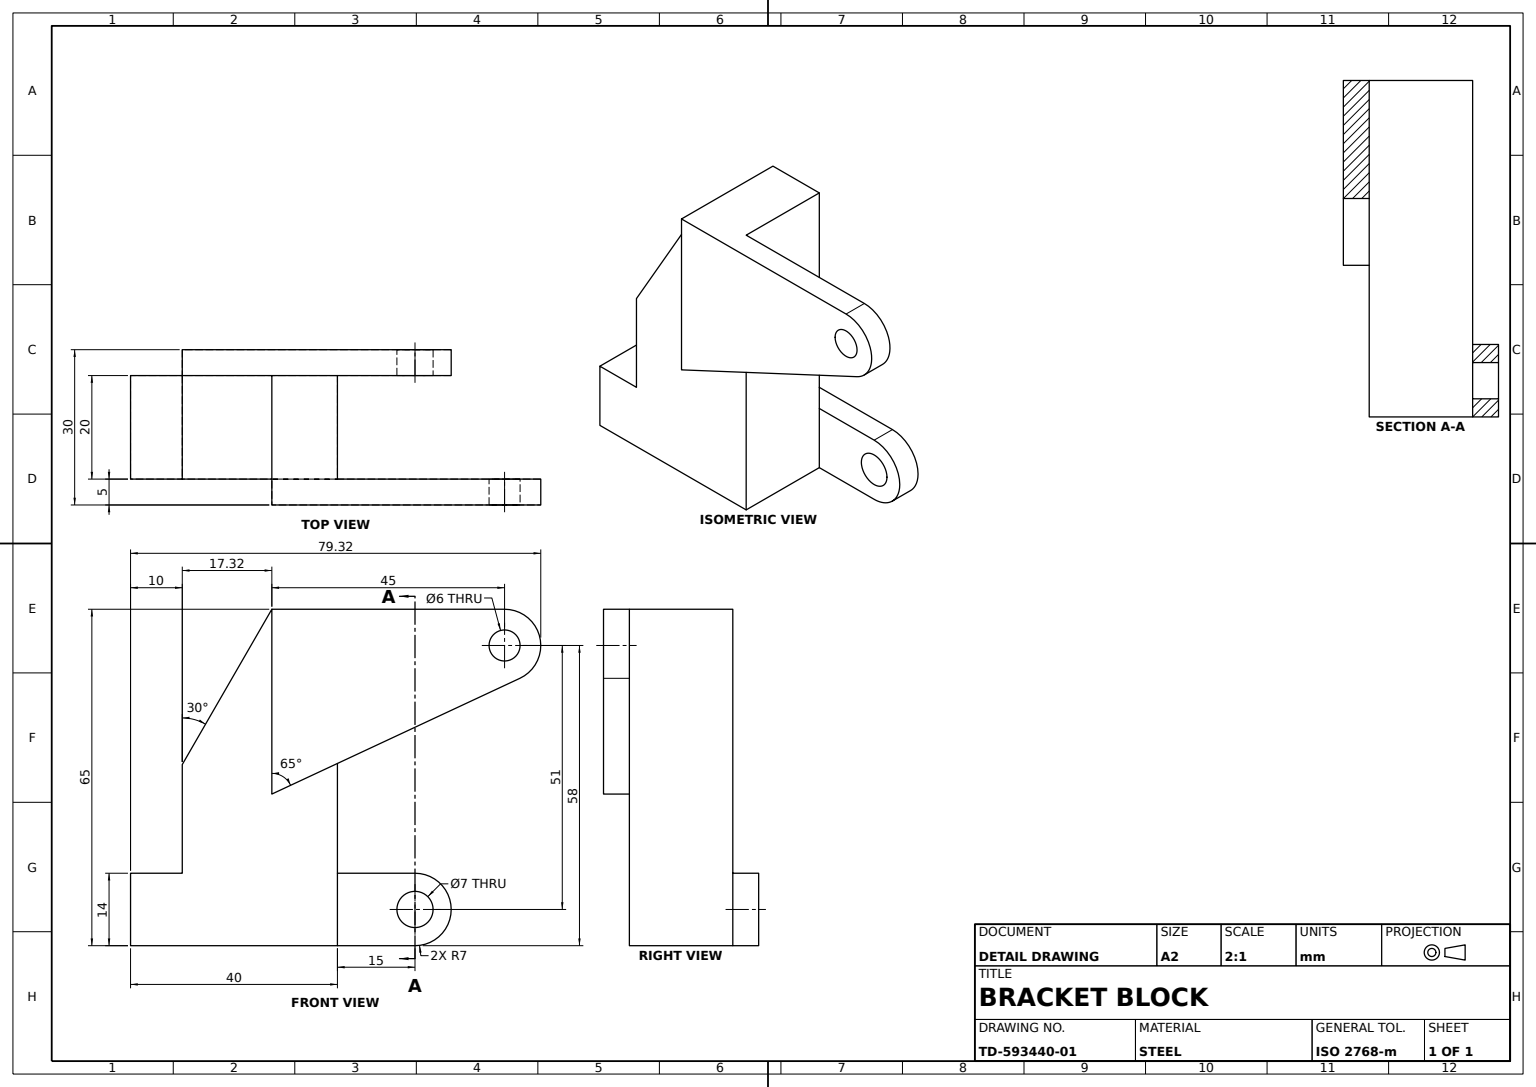
SolidWorks part; units mm, degrees
material "Plain Carbon Steel"
ref_plane "Front Plane" through (0, 0, 0) normal (0, 0, 1) x (1, 0, 0)
ref_plane "Top Plane" through (0, 0, 0) normal (0, 1, 0) x (1, 0, 0)
ref_plane "Right Plane" through (0, 0, 0) normal (1, 0, 0) x (0, 0, -1)
sketch "Base Block Sketch" plane through (0, 0, 0) normal (0, 1, 0) x (1, 0, 0)
  line L1 (0, 0) -> (40, 0)
  line L2 (0, 0) -> (0, -20)
  line L3 (0, -20) -> (40, -20)
  line L4 (40, 0) -> (40, -20)
  dimension "D1" = 40
  dimension "D2" = 20
extrude "Base Block" add sketch "Base Block Sketch" along normal blind 14
sketch "Upright Sketch" plane through (0, 14, 0) normal (0, 1, 0) x (1, 0, 0)
  line L0 (0, -20) -> (40, -20) construction
  line L1 (40, 0) -> (10, 0)
  line L2 (40, 0) -> (40, -20)
  line L3 (40, -20) -> (10, -20)
  line L4 (10, 0) -> (10, -20)
  dimension "D1" = 30
extrude "Upright Block" add sketch "Upright Sketch" along normal blind 51
sketch "Angled Cut Sketch 30deg" plane through (0, 0, 20) normal (0, 0, 1) x (1, 0, 0)
  line L0 (10, 65) -> (10, 35)
  line L1 (40, 65) -> (40, 0) construction
  line L2 (10, 65) -> (10, 14) construction
  line L3 (10, 35) -> (27.3205, 65)
  line L4 (10, 65) -> (40, 65) construction
  line L5 (10, 65) -> (27.3205, 65)
  dimension "D1" = 12.6795
  dimension "D2" = 30
extrude "Angled Cut 30deg" cut sketch "Angled Cut Sketch 30deg" against normal blind 51
sketch "Upper Lug Sketch" plane through (0, 0, 20) normal (0, 0, 1) x (1, 0, 0)
  line L0 (27.3205, 65) -> (27.3205, 29.2925)
  line L1 (27.3205, 29.2925) -> (75.2788, 51.6558)
  line L2 (27.3205, 65) -> (72.3205, 65)
  arc A0 (75.2788, 51.6558) -> (72.3205, 65) centre (72.3205, 58) ccw
  circle A1 centre (72.3205, 58) radius 3
  dimension "D2" = 6
  dimension "D4" = 14
  dimension "D1" = 65
  dimension "D3" = 45
extrude "Upper Lug" add sketch "Upper Lug Sketch" along normal blind 5
sketch "Lower Lug Sketch" plane through (0, 0, 0) normal (0, 0, -1) x (-1, 0, 0)
  line L0 (-40, 65) -> (-40, 0) construction
  line L1 (-10, 14) -> (-55, 14)
  line L2 (-10, 14) -> (-10, 0)
  line L3 (-10, 0) -> (-55, 0)
  arc A0 (-55, 14) -> (-55, 0) centre (-55, 7) ccw
  circle A1 centre (-55, 7) radius 3.5
  dimension "D2" = 7
  dimension "D1" = 7
  dimension "D3" = 15
extrude "Lower Lug" add sketch "Lower Lug Sketch" along normal blind 5
